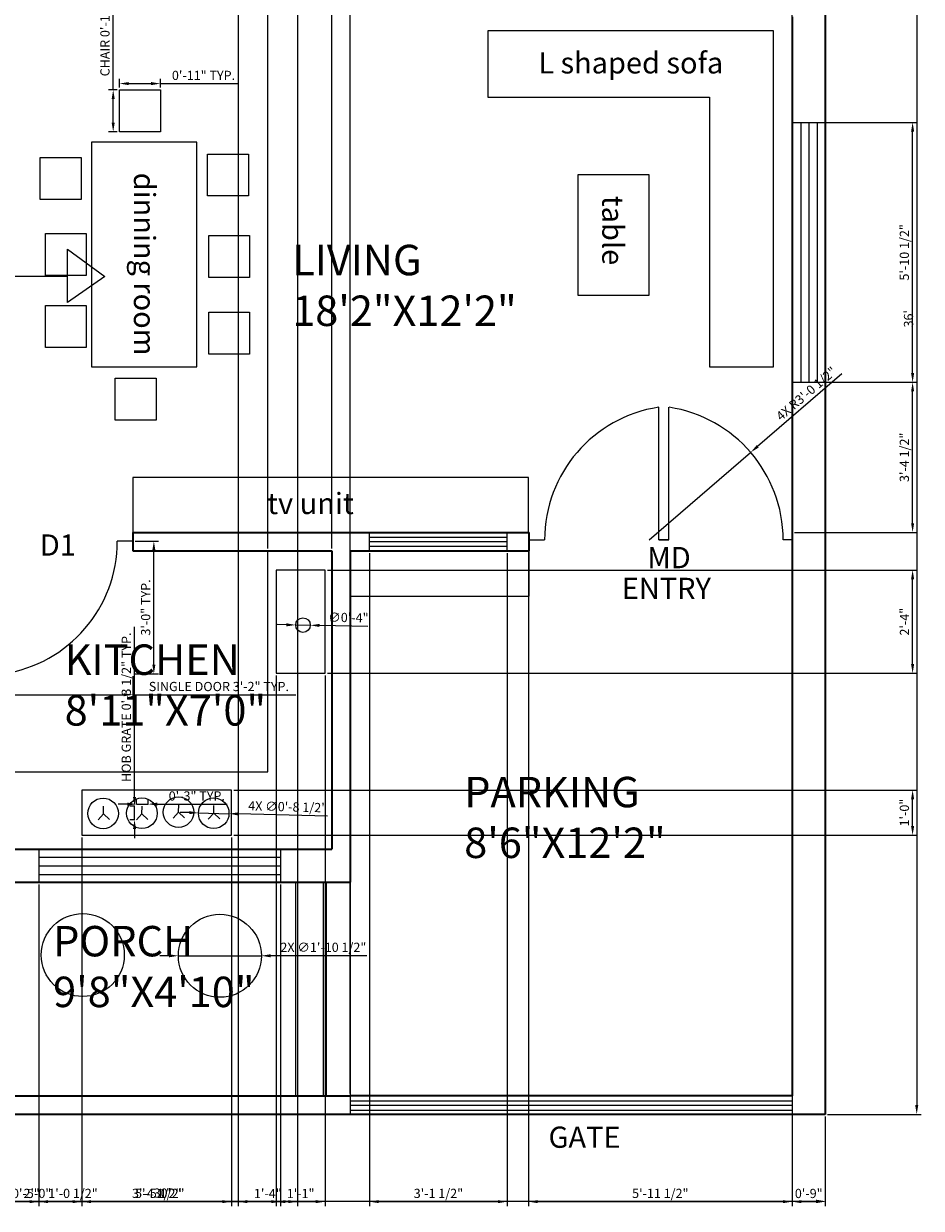
# Model space of a CAD drawing. Units: inches. Extents: x 346 to 762, y 179 to 666.
# Tile 2 of 3: x 518 to 762, y 179 to 500. Entities that reach past the tile are written whole.
import ezdxf

# ---------------------------------------------------------------- set-up
doc = ezdxf.new("R2010")
doc.units = ezdxf.units.IN
for name, color, linetype, lineweight in [('A-ANNO-DIMS', 2, 'Continuous', 18), ('A-ANNO-SYMB', 3, 'Continuous', 18), ('A-ANNO-TEXT', 7, 'Continuous', 18), ('A-AREA-IDEN', 7, 'Continuous', 25), ('A-DOOR', 3, 'Continuous', 25), ('A-EQPM', 8, 'Continuous', 18), ('A-FLOR', 7, 'Continuous', 25), ('A-FLOR-CASE', 9, 'Continuous', 18), ('A-FLOR-FIXT', 9, 'Continuous', 18), ('A-FURN', 8, 'Continuous', 18), ('A-GLAZ', 4, 'Continuous', 18), ('A-WALL', 7, 'Continuous', 35)]:
    doc.layers.add(name, color=color, linetype=linetype, lineweight=lineweight)
doc.styles.get("Standard").update_dxf_attribs({"font": 'arial.ttf'})
doc.dimstyles.new('ISO-25', dxfattribs={"dimtxt": 2.5, "dimasz": 2.5, "dimexe": 1.25, "dimexo": 0.625, "dimtad": 1, "dimdec": 0, "dimlunit": 3, "dimtxsty": 'Standard', "dimcen": 2.5, "dimadec": 0, "dimazin": 0, "dimtfac": 1, "dimtdec": 0, "dimtmove": 0, "dimatfit": 3, "dimfxl": 1, "dimarcsym": 0})

# ---------------------------------------------------------------- blocks, each defined once
blk = doc.blocks.new('*D3')
at = {"layer": 'A-ANNO-DIMS', "color": 0, "lineweight": -2, "transparency": 16777216}
for p, q in [((736.29, 636.22), (761.72, 636.22)), ((760.47, 633.72), (760.47, 206.72)), ((736.29, 204.22), (761.72, 204.22))]:
    blk.add_line(p, q, dxfattribs=at)
at = {"layer": 'A-ANNO-DIMS', "color": 0, "transparency": 16777216}
for points in [[(760.06, 633.72), (760.89, 633.72), (760.47, 636.22)], [(760.06, 206.72), (760.89, 206.72), (760.47, 204.22)]]:
    blk.add_solid(points, dxfattribs=at)
at = {"layer": 'Defpoints', "color": 0, "transparency": 16777216}
for p in [(735.66, 636.22), (735.66, 204.22), (760.47, 204.22)]:
    blk.add_point(p, dxfattribs=at)
at = {"layer": 'A-ANNO-DIMS', "color": 0, "transparency": 16777216, "insert": (758.57, 420.22), "char_height": 2.5, "attachment_point": 5, "rotation": 90}
blk.add_mtext("36'", dxfattribs=at)
blk = doc.blocks.new('*D4')
at = {"layer": 'A-ANNO-DIMS', "color": 0, "lineweight": -2, "transparency": 16777216}
for p, q in [((375.66, 203.6), (375.66, 179.38)), ((735.66, 203.6), (735.66, 179.38)), ((378.16, 180.63), (733.16, 180.63))]:
    blk.add_line(p, q, dxfattribs=at)
at = {"layer": 'A-ANNO-DIMS', "color": 0, "transparency": 16777216}
for points in [[(378.16, 181.05), (378.16, 180.21), (375.66, 180.63)], [(733.16, 181.05), (733.16, 180.21), (735.66, 180.63)]]:
    blk.add_solid(points, dxfattribs=at)
at = {"layer": 'Defpoints', "color": 0, "transparency": 16777216}
for p in [(375.66, 204.22), (735.66, 204.22), (735.66, 180.63)]:
    blk.add_point(p, dxfattribs=at)
at = {"layer": 'A-ANNO-DIMS', "color": 0, "transparency": 16777216, "insert": (555.66, 182.53), "char_height": 2.5, "attachment_point": 5}
blk.add_mtext("30'", dxfattribs=at)
blk = doc.blocks.new('DOOR-SINGLE-36IN')
for p, q in [((2.79, 36), (0, 36)), ((2.79, 36), (2.79, 0)), ((38, 36), (33.78, 36))]:
    blk.add_line(p, q)
blk.add_arc((-2.63, 36), 36.41, 278.5676, 0)
blk = doc.blocks.new('CHAIR-DINING')
blk.add_lwpolyline([(0, 11.39), (11.09, 11.39), (11.09, 0), (0, 0)], close=True)
blk = doc.blocks.new('HOB-PAN-SUPPORT')
for q in [(1.53, 3.67), (0, 0), (3.11, 0.08)]:
    blk.add_line((1.45, 1.6), q)
blk = doc.blocks.new('*D11')
at = {"layer": 'A-ANNO-DIMS', "color": 0, "lineweight": -2, "transparency": 16777216}
for p, q in [((509.66, 323.21), (509.66, 316.88)), ((547.66, 323.21), (547.66, 316.88)), ((512.16, 318.13), (545.16, 318.13)), ((547.66, 318.13), (591.87, 318.13))]:
    blk.add_line(p, q, dxfattribs=at)
at = {"layer": 'A-ANNO-DIMS', "color": 0, "transparency": 16777216}
for points in [[(512.16, 318.55), (512.16, 317.72), (509.66, 318.13)], [(545.16, 318.55), (545.16, 317.72), (547.66, 318.13)]]:
    blk.add_solid(points, dxfattribs=at)
at = {"layer": 'Defpoints', "color": 0, "transparency": 16777216}
for p in [(509.66, 323.83), (547.66, 323.83), (547.66, 318.13)]:
    blk.add_point(p, dxfattribs=at)
at = {"layer": 'A-ANNO-DIMS', "color": 0, "transparency": 16777216, "insert": (571.01, 320.05), "char_height": 2.5, "attachment_point": 5}
blk.add_mtext('SINGLE DOOR 3\'-2" TYP.', dxfattribs=at)
blk = doc.blocks.new('*D12')
at = {"layer": 'A-ANNO-DIMS', "color": 0, "lineweight": -2, "transparency": 16777216}
for p, q in [((548.29, 359.83), (554.61, 359.83)), ((553.36, 326.33), (553.36, 357.33)), ((548.29, 323.83), (554.61, 323.83))]:
    blk.add_line(p, q, dxfattribs=at)
at = {"layer": 'A-ANNO-DIMS', "color": 0, "transparency": 16777216}
for points in [[(552.94, 357.33), (553.78, 357.33), (553.36, 359.83)], [(552.94, 326.33), (553.78, 326.33), (553.36, 323.83)]]:
    blk.add_solid(points, dxfattribs=at)
at = {"layer": 'Defpoints', "color": 0, "transparency": 16777216}
for p in [(547.66, 359.83), (553.36, 359.83), (547.66, 323.83)]:
    blk.add_point(p, dxfattribs=at)
at = {"layer": 'A-ANNO-DIMS', "color": 0, "transparency": 16777216, "insert": (551.46, 341.83), "char_height": 2.5, "attachment_point": 5, "rotation": 90}
blk.add_mtext('3\'-0" TYP.', dxfattribs=at)
blk = doc.blocks.new('*D13')
at = {"layer": 'A-ANNO-DIMS', "color": 0, "lineweight": -2, "transparency": 16777216}
for p, q in [((542.32, 482.35), (542.32, 520.92)), ((543.4, 482.35), (541.07, 482.35)), ((542.32, 473.46), (542.32, 479.85)), ((543.4, 470.96), (541.07, 470.96))]:
    blk.add_line(p, q, dxfattribs=at)
at = {"layer": 'A-ANNO-DIMS', "color": 0, "transparency": 16777216}
for points in [[(541.9, 479.85), (542.74, 479.85), (542.32, 482.35)], [(541.9, 473.46), (542.74, 473.46), (542.32, 470.96)]]:
    blk.add_solid(points, dxfattribs=at)
at = {"layer": 'Defpoints', "color": 0, "transparency": 16777216}
for p in [(542.32, 482.35), (544.03, 482.35), (544.03, 470.96)]:
    blk.add_point(p, dxfattribs=at)
at = {"layer": 'A-ANNO-DIMS', "color": 0, "transparency": 16777216, "insert": (540.4, 502.88), "char_height": 2.5, "attachment_point": 5, "rotation": 90}
blk.add_mtext('CHAIR 0\'-11 1/2" TYP.', dxfattribs=at)
blk = doc.blocks.new('*D14')
at = {"layer": 'A-ANNO-DIMS', "color": 0, "lineweight": -2, "transparency": 16777216}
for p, q in [((544.03, 482.98), (544.03, 485.31)), ((546.53, 484.06), (552.62, 484.06)), ((555.12, 482.98), (555.12, 485.31)), ((555.12, 484.06), (576.05, 484.06))]:
    blk.add_line(p, q, dxfattribs=at)
at = {"layer": 'A-ANNO-DIMS', "color": 0, "transparency": 16777216}
for points in [[(546.53, 484.48), (546.53, 483.64), (544.03, 484.06)], [(552.62, 484.48), (552.62, 483.64), (555.12, 484.06)]]:
    blk.add_solid(points, dxfattribs=at)
at = {"layer": 'Defpoints', "color": 0, "transparency": 16777216}
for p in [(555.12, 484.06), (544.03, 482.35), (555.12, 482.35)]:
    blk.add_point(p, dxfattribs=at)
at = {"layer": 'A-ANNO-DIMS', "color": 0, "transparency": 16777216, "insert": (566.84, 485.96), "char_height": 2.5, "attachment_point": 5}
blk.add_mtext('0\'-11" TYP.', dxfattribs=at)
blk = doc.blocks.new('*D15')
at = {"layer": 'A-ANNO-DIMS', "color": 0, "lineweight": -2, "transparency": 16777216}
for p, q in [((548.11, 290.39), (548.11, 336.61)), ((548.04, 287.89), (546.86, 287.89)), ((548.11, 284.22), (548.11, 287.89)), ((548.04, 284.22), (546.86, 284.22)), ((548.11, 281.72), (548.11, 279.22))]:
    blk.add_line(p, q, dxfattribs=at)
at = {"layer": 'A-ANNO-DIMS', "color": 0, "transparency": 16777216}
for points in [[(547.7, 290.39), (548.53, 290.39), (548.11, 287.89)], [(547.7, 281.72), (548.53, 281.72), (548.11, 284.22)]]:
    blk.add_solid(points, dxfattribs=at)
at = {"layer": 'Defpoints', "color": 0, "transparency": 16777216}
for p in [(548.11, 287.89), (548.66, 287.89), (548.66, 284.22)]:
    blk.add_point(p, dxfattribs=at)
at = {"layer": 'A-ANNO-DIMS', "color": 0, "transparency": 16777216, "insert": (546.19, 314.75), "char_height": 2.5, "attachment_point": 5, "rotation": 90}
blk.add_mtext('HOB GRATE 0\'-3 1/2" TYP.', dxfattribs=at)
blk = doc.blocks.new('*D16')
at = {"layer": 'A-ANNO-DIMS', "color": 0, "lineweight": -2, "transparency": 16777216}
for p, q in [((548.66, 288.51), (548.66, 289.69)), ((551.78, 288.51), (551.78, 289.69)), ((546.16, 288.44), (543.66, 288.44)), ((548.66, 288.44), (551.78, 288.44)), ((554.28, 288.44), (573.26, 288.44))]:
    blk.add_line(p, q, dxfattribs=at)
at = {"layer": 'A-ANNO-DIMS', "color": 0, "transparency": 16777216}
for points in [[(546.16, 288.86), (546.16, 288.02), (548.66, 288.44)], [(554.28, 288.86), (554.28, 288.02), (551.78, 288.44)]]:
    blk.add_solid(points, dxfattribs=at)
at = {"layer": 'Defpoints', "color": 0, "transparency": 16777216}
for p in [(548.66, 287.89), (551.78, 288.44), (551.78, 287.89)]:
    blk.add_point(p, dxfattribs=at)
at = {"layer": 'A-ANNO-DIMS', "color": 0, "transparency": 16777216, "insert": (565.02, 290.34), "char_height": 2.5, "attachment_point": 5}
blk.add_mtext('0\'-3" TYP.', dxfattribs=at)
blk = doc.blocks.new('*D18')
at = {"layer": 'A-ANNO-DIMS', "color": 0, "lineweight": -2, "transparency": 16777216}
for p, q in [((584.3, 357.85), (584.3, 661.17)), ((586.8, 659.92), (599.16, 659.92)), ((601.66, 357.85), (601.66, 661.17))]:
    blk.add_line(p, q, dxfattribs=at)
at = {"layer": 'A-ANNO-DIMS', "color": 0, "transparency": 16777216}
for points in [[(586.8, 660.34), (586.8, 659.51), (584.3, 659.92)], [(599.16, 660.34), (599.16, 659.51), (601.66, 659.92)]]:
    blk.add_solid(points, dxfattribs=at)
at = {"layer": 'Defpoints', "color": 0, "transparency": 16777216}
for p in [(601.66, 659.92), (584.3, 357.22), (601.66, 357.22)]:
    blk.add_point(p, dxfattribs=at)
at = {"layer": 'A-ANNO-DIMS', "color": 0, "transparency": 16777216, "insert": (592.98, 661.84), "char_height": 2.5, "attachment_point": 5}
blk.add_mtext('1\'-5 1/2"', dxfattribs=at)
blk = doc.blocks.new('*D19')
at = {"layer": 'A-ANNO-DIMS', "color": 0, "lineweight": -2, "transparency": 16777216}
for p, q in [((533.83, 279.4), (533.83, 179.27)), ((509.66, 275.6), (509.66, 179.27)), ((512.16, 180.52), (531.33, 180.52))]:
    blk.add_line(p, q, dxfattribs=at)
at = {"layer": 'A-ANNO-DIMS', "color": 0, "transparency": 16777216}
for points in [[(512.16, 180.94), (512.16, 180.11), (509.66, 180.52)], [(531.33, 180.94), (531.33, 180.11), (533.83, 180.52)]]:
    blk.add_solid(points, dxfattribs=at)
at = {"layer": 'Defpoints', "color": 0, "transparency": 16777216}
for p in [(533.83, 280.02), (509.66, 276.22), (533.83, 180.52)]:
    blk.add_point(p, dxfattribs=at)
at = {"layer": 'A-ANNO-DIMS', "color": 0, "transparency": 16777216, "insert": (521.75, 182.42), "char_height": 2.5, "attachment_point": 5}
blk.add_mtext('2\'-0"', dxfattribs=at)
blk = doc.blocks.new('*D20')
at = {"layer": 'A-ANNO-DIMS', "color": 0, "lineweight": -2, "transparency": 16777216}
for p, q in [((533.83, 279.4), (533.83, 179.27)), ((574.44, 279.4), (574.44, 179.27)), ((536.33, 180.52), (571.94, 180.52))]:
    blk.add_line(p, q, dxfattribs=at)
at = {"layer": 'A-ANNO-DIMS', "color": 0, "transparency": 16777216}
for points in [[(536.33, 180.94), (536.33, 180.11), (533.83, 180.52)], [(571.94, 180.94), (571.94, 180.11), (574.44, 180.52)]]:
    blk.add_solid(points, dxfattribs=at)
at = {"layer": 'Defpoints', "color": 0, "transparency": 16777216}
for p in [(533.83, 280.02), (574.44, 280.02), (574.44, 180.52)]:
    blk.add_point(p, dxfattribs=at)
at = {"layer": 'A-ANNO-DIMS', "color": 0, "transparency": 16777216, "insert": (554.13, 182.44), "char_height": 2.5, "attachment_point": 5}
blk.add_mtext('3\'-4 1/2"', dxfattribs=at)
blk = doc.blocks.new('*D21')
at = {"layer": 'A-ANNO-DIMS', "color": 0, "lineweight": -2, "transparency": 16777216}
for p, q in [((575.06, 292.27), (760.61, 292.27)), ((759.36, 282.52), (759.36, 289.77)), ((575.06, 280.02), (760.61, 280.02))]:
    blk.add_line(p, q, dxfattribs=at)
at = {"layer": 'A-ANNO-DIMS', "color": 0, "transparency": 16777216}
for points in [[(758.94, 289.77), (759.78, 289.77), (759.36, 292.27)], [(758.94, 282.52), (759.78, 282.52), (759.36, 280.02)]]:
    blk.add_solid(points, dxfattribs=at)
at = {"layer": 'Defpoints', "color": 0, "transparency": 16777216}
for p in [(574.44, 292.27), (759.36, 292.27), (574.44, 280.02)]:
    blk.add_point(p, dxfattribs=at)
at = {"layer": 'A-ANNO-DIMS', "color": 0, "transparency": 16777216, "insert": (757.46, 286.15), "char_height": 2.5, "attachment_point": 5, "rotation": 90}
blk.add_mtext('1\'-0"', dxfattribs=at)
blk = doc.blocks.new('*D22')
at = {"layer": 'A-ANNO-DIMS', "color": 0, "lineweight": -2, "transparency": 16777216}
for p, q in [((600.46, 351.98), (760.61, 351.98)), ((759.36, 326.47), (759.36, 349.48)), ((600.46, 323.97), (760.61, 323.97))]:
    blk.add_line(p, q, dxfattribs=at)
at = {"layer": 'A-ANNO-DIMS', "color": 0, "transparency": 16777216}
for points in [[(758.94, 349.48), (759.78, 349.48), (759.36, 351.98)], [(758.94, 326.47), (759.78, 326.47), (759.36, 323.97)]]:
    blk.add_solid(points, dxfattribs=at)
at = {"layer": 'Defpoints', "color": 0, "transparency": 16777216}
for p in [(599.83, 351.98), (759.36, 351.98), (599.83, 323.97)]:
    blk.add_point(p, dxfattribs=at)
at = {"layer": 'A-ANNO-DIMS', "color": 0, "transparency": 16777216, "insert": (757.48, 337.97), "char_height": 2.5, "attachment_point": 5, "rotation": 90}
blk.add_mtext('2\'-4"', dxfattribs=at)
blk = doc.blocks.new('*D23')
at = {"layer": 'A-ANNO-DIMS', "color": 0, "lineweight": -2, "transparency": 16777216}
for p, q in [((586.58, 323.34), (586.58, 179.27)), ((599.83, 323.34), (599.83, 179.27)), ((589.08, 180.52), (597.33, 180.52))]:
    blk.add_line(p, q, dxfattribs=at)
at = {"layer": 'A-ANNO-DIMS', "color": 0, "transparency": 16777216}
for points in [[(589.08, 180.94), (589.08, 180.11), (586.58, 180.52)], [(597.33, 180.94), (597.33, 180.11), (599.83, 180.52)]]:
    blk.add_solid(points, dxfattribs=at)
at = {"layer": 'Defpoints', "color": 0, "transparency": 16777216}
for p in [(586.58, 323.97), (599.83, 323.97), (599.83, 180.52)]:
    blk.add_point(p, dxfattribs=at)
at = {"layer": 'A-ANNO-DIMS', "color": 0, "transparency": 16777216, "insert": (593.21, 182.4), "char_height": 2.5, "attachment_point": 5}
blk.add_mtext('1\'-1"', dxfattribs=at)
blk = doc.blocks.new('*D24')
at = {"layer": 'A-ANNO-DIMS', "color": 0, "lineweight": -2, "transparency": 16777216}
for p, q in [((509.66, 266.6), (509.66, 179.27)), ((522.15, 266.6), (522.15, 179.27)), ((512.16, 180.52), (519.65, 180.52)), ((522.15, 180.52), (538.14, 180.52))]:
    blk.add_line(p, q, dxfattribs=at)
at = {"layer": 'A-ANNO-DIMS', "color": 0, "transparency": 16777216}
for points in [[(512.16, 180.94), (512.16, 180.11), (509.66, 180.52)], [(519.65, 180.94), (519.65, 180.11), (522.15, 180.52)]]:
    blk.add_solid(points, dxfattribs=at)
at = {"layer": 'Defpoints', "color": 0, "transparency": 16777216}
for p in [(509.66, 267.22), (522.15, 267.22), (522.15, 180.52)]:
    blk.add_point(p, dxfattribs=at)
at = {"layer": 'A-ANNO-DIMS', "color": 0, "transparency": 16777216, "insert": (531.4, 182.44), "char_height": 2.5, "attachment_point": 5}
blk.add_mtext('1\'-0 1/2"', dxfattribs=at)
blk = doc.blocks.new('*D25')
at = {"layer": 'A-ANNO-DIMS', "color": 0, "lineweight": -2, "transparency": 16777216}
for p, q in [((522.15, 266.6), (522.15, 179.27)), ((587.77, 266.6), (587.77, 179.27)), ((524.65, 180.52), (585.27, 180.52))]:
    blk.add_line(p, q, dxfattribs=at)
at = {"layer": 'A-ANNO-DIMS', "color": 0, "transparency": 16777216}
for points in [[(524.65, 180.94), (524.65, 180.11), (522.15, 180.52)], [(585.27, 180.94), (585.27, 180.11), (587.77, 180.52)]]:
    blk.add_solid(points, dxfattribs=at)
at = {"layer": 'Defpoints', "color": 0, "transparency": 16777216}
for p in [(522.15, 267.22), (587.77, 267.22), (587.77, 180.52)]:
    blk.add_point(p, dxfattribs=at)
at = {"layer": 'A-ANNO-DIMS', "color": 0, "transparency": 16777216, "insert": (554.96, 182.44), "char_height": 2.5, "attachment_point": 5}
blk.add_mtext('5\'-5 1/2"', dxfattribs=at)
blk = doc.blocks.new('*D37')
at = {"layer": 'A-ANNO-DIMS', "color": 0, "lineweight": -2, "transparency": 16777216}
for p, q in [((727.29, 473.5), (760.61, 473.5)), ((759.36, 405.47), (759.36, 471)), ((727.29, 402.97), (760.61, 402.97))]:
    blk.add_line(p, q, dxfattribs=at)
at = {"layer": 'A-ANNO-DIMS', "color": 0, "transparency": 16777216}
for points in [[(758.94, 471), (759.78, 471), (759.36, 473.5)], [(758.94, 405.47), (759.78, 405.47), (759.36, 402.97)]]:
    blk.add_solid(points, dxfattribs=at)
at = {"layer": 'Defpoints', "color": 0, "transparency": 16777216}
for p in [(726.66, 473.5), (759.36, 473.5), (726.66, 402.97)]:
    blk.add_point(p, dxfattribs=at)
at = {"layer": 'A-ANNO-DIMS', "color": 0, "transparency": 16777216, "insert": (757.44, 438.24), "char_height": 2.5, "attachment_point": 5, "rotation": 90}
blk.add_mtext('5\'-10 1/2"', dxfattribs=at)
blk = doc.blocks.new('*D38')
at = {"layer": 'A-ANNO-DIMS', "color": 0, "lineweight": -2, "transparency": 16777216}
for p, q in [((727.29, 402.97), (760.61, 402.97)), ((759.36, 364.72), (759.36, 400.47)), ((727.29, 362.22), (760.61, 362.22))]:
    blk.add_line(p, q, dxfattribs=at)
at = {"layer": 'A-ANNO-DIMS', "color": 0, "transparency": 16777216}
for points in [[(758.94, 400.47), (759.78, 400.47), (759.36, 402.97)], [(758.94, 364.72), (759.78, 364.72), (759.36, 362.22)]]:
    blk.add_solid(points, dxfattribs=at)
at = {"layer": 'Defpoints', "color": 0, "transparency": 16777216}
for p in [(726.66, 402.97), (759.36, 402.97), (726.66, 362.22)]:
    blk.add_point(p, dxfattribs=at)
at = {"layer": 'A-ANNO-DIMS', "color": 0, "transparency": 16777216, "insert": (757.44, 382.6), "char_height": 2.5, "attachment_point": 5, "rotation": 90}
blk.add_mtext('3\'-4 1/2"', dxfattribs=at)
blk = doc.blocks.new('*D39')
at = {"layer": 'A-ANNO-DIMS', "color": 0, "lineweight": -2, "transparency": 16777216}
for p, q in [((606.66, 209.85), (606.66, 661.17)), ((609.16, 659.92), (724.16, 659.92)), ((726.66, 209.85), (726.66, 661.17))]:
    blk.add_line(p, q, dxfattribs=at)
at = {"layer": 'A-ANNO-DIMS', "color": 0, "transparency": 16777216}
for points in [[(609.16, 660.34), (609.16, 659.51), (606.66, 659.92)], [(724.16, 660.34), (724.16, 659.51), (726.66, 659.92)]]:
    blk.add_solid(points, dxfattribs=at)
at = {"layer": 'Defpoints', "color": 0, "transparency": 16777216}
for p in [(726.66, 659.92), (606.66, 209.22), (726.66, 209.22)]:
    blk.add_point(p, dxfattribs=at)
at = {"layer": 'A-ANNO-DIMS', "color": 0, "transparency": 16777216, "insert": (666.66, 661.82), "char_height": 2.5, "attachment_point": 5}
blk.add_mtext('10\'-0"', dxfattribs=at)
blk = doc.blocks.new('*D40')
at = {"layer": 'A-ANNO-DIMS', "color": 0, "lineweight": -2, "transparency": 16777216}
for p, q in [((726.66, 208.6), (726.66, 179.27)), ((735.66, 203.6), (735.66, 179.27)), ((729.16, 180.52), (733.16, 180.52))]:
    blk.add_line(p, q, dxfattribs=at)
at = {"layer": 'A-ANNO-DIMS', "color": 0, "transparency": 16777216}
for points in [[(729.16, 180.94), (729.16, 180.11), (726.66, 180.52)], [(733.16, 180.94), (733.16, 180.11), (735.66, 180.52)]]:
    blk.add_solid(points, dxfattribs=at)
at = {"layer": 'Defpoints', "color": 0, "transparency": 16777216}
for p in [(726.66, 209.22), (735.66, 204.22), (735.66, 180.52)]:
    blk.add_point(p, dxfattribs=at)
at = {"layer": 'A-ANNO-DIMS', "color": 0, "transparency": 16777216, "insert": (731.16, 182.42), "char_height": 2.5, "attachment_point": 5}
blk.add_mtext('0\'-9"', dxfattribs=at)
blk = doc.blocks.new('*D43')
at = {"layer": 'A-ANNO-DIMS', "color": 0, "lineweight": -2, "transparency": 16777216}
for p, q in [((611.94, 356.6), (611.94, 179.27)), ((649.31, 356.6), (649.31, 179.27)), ((614.44, 180.52), (646.81, 180.52))]:
    blk.add_line(p, q, dxfattribs=at)
at = {"layer": 'A-ANNO-DIMS', "color": 0, "transparency": 16777216}
for points in [[(614.44, 180.94), (614.44, 180.11), (611.94, 180.52)], [(646.81, 180.94), (646.81, 180.11), (649.31, 180.52)]]:
    blk.add_solid(points, dxfattribs=at)
at = {"layer": 'Defpoints', "color": 0, "transparency": 16777216}
for p in [(611.94, 357.22), (649.31, 357.22), (649.31, 180.52)]:
    blk.add_point(p, dxfattribs=at)
at = {"layer": 'A-ANNO-DIMS', "color": 0, "transparency": 16777216, "insert": (630.62, 182.44), "char_height": 2.5, "attachment_point": 5}
blk.add_mtext('3\'-1 1/2"', dxfattribs=at)
blk = doc.blocks.new('*D44')
at = {"layer": 'A-ANNO-DIMS', "color": 0, "lineweight": -2, "transparency": 16777216}
for p, q in [((655.05, 361.6), (655.05, 179.27)), ((726.66, 361.6), (726.66, 179.27)), ((657.55, 180.52), (724.16, 180.52))]:
    blk.add_line(p, q, dxfattribs=at)
at = {"layer": 'A-ANNO-DIMS', "color": 0, "transparency": 16777216}
for points in [[(657.55, 180.94), (657.55, 180.11), (655.05, 180.52)], [(724.16, 180.94), (724.16, 180.11), (726.66, 180.52)]]:
    blk.add_solid(points, dxfattribs=at)
at = {"layer": 'Defpoints', "color": 0, "transparency": 16777216}
for p in [(655.05, 362.22), (726.66, 362.22), (726.66, 180.52)]:
    blk.add_point(p, dxfattribs=at)
at = {"layer": 'A-ANNO-DIMS', "color": 0, "transparency": 16777216, "insert": (690.86, 182.44), "char_height": 2.5, "attachment_point": 5}
blk.add_mtext('5\'-11 1/2"', dxfattribs=at)
blk = doc.blocks.new('*D46')
at = {"layer": 'A-ANNO-DIMS', "color": 0, "lineweight": -2, "transparency": 16777216}
for p, q in [((576.21, 585.6), (576.21, 179.27)), ((592.38, 585.6), (592.38, 179.27)), ((578.71, 180.52), (589.88, 180.52))]:
    blk.add_line(p, q, dxfattribs=at)
at = {"layer": 'A-ANNO-DIMS', "color": 0, "transparency": 16777216}
for points in [[(578.71, 180.94), (578.71, 180.11), (576.21, 180.52)], [(589.88, 180.94), (589.88, 180.11), (592.38, 180.52)]]:
    blk.add_solid(points, dxfattribs=at)
at = {"layer": 'Defpoints', "color": 0, "transparency": 16777216}
for p in [(576.21, 586.22), (592.38, 586.22), (592.38, 180.52)]:
    blk.add_point(p, dxfattribs=at)
at = {"layer": 'A-ANNO-DIMS', "color": 0, "transparency": 16777216, "insert": (584.3, 182.4), "char_height": 2.5, "attachment_point": 5}
blk.add_mtext('1\'-4"', dxfattribs=at)
blk = doc.blocks.new('*D47')
at = {"layer": 'A-ANNO-DIMS', "color": 0, "lineweight": -2, "transparency": 16777216}
for p, q in [((504.66, 236.6), (504.66, 179.27)), ((509.66, 231.6), (509.66, 179.27)), ((502.16, 180.52), (499.66, 180.52)), ((504.66, 180.52), (509.66, 180.52)), ((512.16, 180.52), (522.56, 180.52))]:
    blk.add_line(p, q, dxfattribs=at)
at = {"layer": 'A-ANNO-DIMS', "color": 0, "transparency": 16777216}
for points in [[(502.16, 180.94), (502.16, 180.11), (504.66, 180.52)], [(512.16, 180.94), (512.16, 180.11), (509.66, 180.52)]]:
    blk.add_solid(points, dxfattribs=at)
at = {"layer": 'Defpoints', "color": 0, "transparency": 16777216}
for p in [(504.66, 237.22), (509.66, 232.22), (509.66, 180.52)]:
    blk.add_point(p, dxfattribs=at)
at = {"layer": 'A-ANNO-DIMS', "color": 0, "transparency": 16777216, "insert": (518.61, 182.42), "char_height": 2.5, "attachment_point": 5}
blk.add_mtext('0\'-5"', dxfattribs=at)
blk = doc.blocks.new('*D48')
at = {"layer": 'A-ANNO-DIMS', "color": 0, "lineweight": -2, "transparency": 16777216}
for p, q in [((740.13, 405.22), (717.29, 385.56)), ((687.8, 360.18), (715.39, 383.93))]:
    blk.add_line(p, q, dxfattribs=at)
at = {"layer": 'A-ANNO-DIMS', "color": 0, "transparency": 16777216}
blk.add_solid([(717.02, 385.88), (717.56, 385.25), (715.39, 383.93)], dxfattribs=at)
at = {"layer": 'Defpoints', "color": 0, "transparency": 16777216}
for p in [(715.39, 383.93), (687.8, 360.18)]:
    blk.add_point(p, dxfattribs=at)
at = {"layer": 'A-ANNO-DIMS', "color": 0, "transparency": 16777216, "insert": (730.7, 399.63), "char_height": 2.5, "attachment_point": 5, "rotation": 40.716}
blk.add_mtext('4X R3\'-0 1/2"', dxfattribs=at)
blk = doc.blocks.new('*D49')
at = {"layer": 'A-ANNO-DIMS', "color": 0, "lineweight": -2, "transparency": 16777216}
for p, q in [((557.51, 247.27), (555.01, 247.27)), ((560.01, 247.27), (582.54, 247.27)), ((611.21, 247.27), (585.04, 247.27))]:
    blk.add_line(p, q, dxfattribs=at)
at = {"layer": 'A-ANNO-DIMS', "color": 0, "transparency": 16777216}
for points in [[(557.51, 247.69), (557.51, 246.86), (560.01, 247.27)], [(585.04, 247.69), (585.04, 246.86), (582.54, 247.27)]]:
    blk.add_solid(points, dxfattribs=at)
at = {"layer": 'Defpoints', "color": 0, "transparency": 16777216}
for p in [(560.01, 247.27), (582.54, 247.27)]:
    blk.add_point(p, dxfattribs=at)
at = {"layer": 'A-ANNO-DIMS', "color": 0, "transparency": 16777216, "insert": (599.38, 249.25), "char_height": 2.5, "attachment_point": 5, "rotation": 0.0023}
blk.add_mtext('2X ∅1\'-10 1/2"', dxfattribs=at)
blk = doc.blocks.new('*D51')
at = {"layer": 'A-ANNO-DIMS', "color": 0, "lineweight": -2, "transparency": 16777216}
for p, q in [((589.37, 337.12), (586.87, 337.17)), ((591.87, 337.08), (595.83, 337)), ((611.44, 336.7), (598.33, 336.95))]:
    blk.add_line(p, q, dxfattribs=at)
at = {"layer": 'A-ANNO-DIMS', "color": 0, "transparency": 16777216}
for points in [[(589.37, 337.54), (589.36, 336.71), (591.87, 337.08)], [(598.34, 337.37), (598.32, 336.54), (595.83, 337)]]:
    blk.add_solid(points, dxfattribs=at)
at = {"layer": 'Defpoints', "color": 0, "transparency": 16777216}
for p in [(591.87, 337.08), (595.83, 337)]:
    blk.add_point(p, dxfattribs=at)
at = {"layer": 'A-ANNO-DIMS', "color": 0, "transparency": 16777216, "insert": (606.17, 338.77), "char_height": 2.5, "attachment_point": 5, "rotation": 358.898}
blk.add_mtext('∅0\'-4"', dxfattribs=at)
blk = doc.blocks.new('*D52')
at = {"layer": 'A-ANNO-DIMS', "color": 0, "lineweight": -2, "transparency": 16777216}
for p, q in [((562.96, 286.13), (560.46, 286.2)), ((565.46, 286.06), (573.76, 285.85)), ((600.53, 285.15), (576.26, 285.78))]:
    blk.add_line(p, q, dxfattribs=at)
at = {"layer": 'A-ANNO-DIMS', "color": 0, "transparency": 16777216}
for points in [[(562.97, 286.55), (562.95, 285.71), (565.46, 286.06)], [(576.27, 286.2), (576.25, 285.37), (573.76, 285.85)]]:
    blk.add_solid(points, dxfattribs=at)
at = {"layer": 'Defpoints', "color": 0, "transparency": 16777216}
for p in [(565.46, 286.06), (573.76, 285.85)]:
    blk.add_point(p, dxfattribs=at)
at = {"layer": 'A-ANNO-DIMS', "color": 0, "transparency": 16777216, "insert": (589.69, 287.4), "char_height": 2.5, "attachment_point": 5, "rotation": 358.5022}
blk.add_mtext('4X ∅0\'-8 1/2"', dxfattribs=at)

msp = doc.modelspace()

# ---------------------------------------------------------------- linework, layer by layer
at = {"layer": 'A-ANNO-SYMB'}
for p, q in [((529.92, 431.72), (529.92, 439.12)), ((529.92, 439.12), (540.07, 431.72)), ((529.92, 431.72), (402.56, 431.72)), ((540.07, 431.72), (529.92, 424.62)), ((529.92, 424.62), (529.92, 431.72))]:
    msp.add_line(p, q, dxfattribs=at)
at = {"layer": 'A-DOOR'}
for p, q in [((690.43, 360.18), (690.43, 396.18)), ((693.22, 360.18), (693.22, 396.18)), ((655.22, 360.18), (659.45, 360.18)), ((690.43, 360.18), (693.22, 360.18)), ((693.22, 360.18), (690.43, 360.18)), ((726.66, 360.18), (724.21, 360.18)), ((606.66, 209.22), (606.66, 204.22)), ((726.66, 209.22), (726.66, 204.22)), ((606.66, 207.89), (726.66, 207.89)), ((606.66, 206.72), (726.66, 206.72)), ((606.66, 205.35), (726.66, 205.35))]:
    msp.add_line(p, q, dxfattribs=at)
for centre, start, end in [((695.85, 360.18), 98.5676, 180), ((687.8, 360.18), 0, 81.4324)]:
    msp.add_arc(centre, 36.41, start, end, dxfattribs=at)
at = {"layer": 'A-EQPM'}
msp.add_lwpolyline([(533.83, 280.02), (574.44, 280.02), (574.44, 292.27), (533.83, 292.27)], close=True, dxfattribs=at)
for centre in [(539.58, 285.92), (550.12, 285.96), (560.05, 286.26), (569.61, 285.96)]:
    msp.add_circle(centre, 4.15, dxfattribs=at)
at = {"layer": 'A-FLOR'}
for p, q in [((591.86, 267.22), (591.86, 209.22)), ((599.37, 267.22), (599.37, 209.22)), ((600.14, 267.22), (600.14, 209.22)), ((606.66, 267.22), (606.66, 209.22))]:
    msp.add_line(p, q, dxfattribs=at)
msp.add_lwpolyline([(655.22, 357.22), (606.66, 357.22), (606.66, 344.87), (655.22, 344.87)], close=True, dxfattribs=at)
at = {"layer": 'A-FLOR-CASE'}
for p, q in [((584.3, 297.23), (584.3, 357.22)), ((509.66, 297.23), (584.3, 297.23))]:
    msp.add_line(p, q, dxfattribs=at)
msp.add_lwpolyline([(547.66, 362.22), (655.05, 362.22), (655.05, 377.14), (547.66, 377.14)], close=True, dxfattribs=at)
at = {"layer": 'A-FLOR-FIXT'}
for p, q in [((586.58, 351.98), (586.58, 323.97)), ((599.83, 351.98), (586.58, 351.98)), ((599.83, 323.97), (599.83, 351.98)), ((586.58, 323.97), (599.83, 323.97))]:
    msp.add_line(p, q, dxfattribs=at)
msp.add_circle((593.85, 337.04), 1.98, dxfattribs=at)
at = {"layer": 'A-FURN'}
for points in [[(721.6, 480.33), (721.6, 498.42), (643.99, 498.42), (643.99, 480.33), (704.26, 480.33)], [(704.26, 480.33), (704.26, 407.16), (721.6, 407.16), (721.6, 498.42), (704.26, 498.42)]]:
    msp.add_lwpolyline(points, dxfattribs=at)
for points in [[(536.47, 407.16), (565.04, 407.16), (565.04, 468.15), (536.47, 468.15)], [(668.56, 459.38), (687.71, 459.38), (687.71, 426.55), (668.56, 426.55)]]:
    msp.add_lwpolyline(points, close=True, dxfattribs=at)
for centre in [(534.06, 247.48), (571.28, 247.27)]:
    msp.add_circle(centre, 11.27, dxfattribs=at)
at = {"layer": 'A-GLAZ'}
for p, q in [((726.66, 473.5), (735.66, 473.5)), ((729.04, 473.5), (729.04, 402.97)), ((731.16, 473.5), (731.16, 402.97)), ((733.43, 473.5), (733.43, 402.97)), ((726.66, 402.97), (735.66, 402.97)), ((611.94, 357.22), (611.94, 362.22)), ((611.94, 360.93), (649.31, 360.93)), ((649.31, 357.22), (649.31, 362.22)), ((611.94, 359.72), (649.31, 359.72)), ((611.94, 358.46), (649.31, 358.46)), ((522.15, 276.22), (522.15, 267.22)), ((522.15, 274.01), (587.77, 274.01)), ((587.77, 276.22), (587.77, 267.22)), ((522.15, 271.72), (587.77, 271.72)), ((522.15, 269.31), (587.77, 269.31))]:
    msp.add_line(p, q, dxfattribs=at)
at = {"layer": 'A-WALL'}
for p, q in [((735.66, 636.22), (735.66, 204.22)), ((726.66, 502.22), (726.66, 362.22)), ((547.66, 362.22), (655.22, 362.22)), ((547.66, 362.22), (547.66, 357.22)), ((655.22, 357.22), (655.22, 362.22)), ((726.66, 362.22), (726.66, 209.22)), ((547.66, 357.22), (601.66, 357.22)), ((601.66, 357.22), (601.66, 276.22)), ((606.66, 357.22), (606.66, 267.22)), ((606.66, 357.22), (655.22, 357.22)), ((509.66, 276.22), (601.66, 276.22)), ((509.66, 267.22), (606.66, 267.22)), ((509.66, 209.22), (606.66, 209.22)), ((726.66, 209.22), (606.66, 209.22)), ((735.66, 204.22), (375.66, 204.22))]:
    msp.add_line(p, q, dxfattribs=at)

# ---------------------------------------------------------------- block references
at = {"layer": 'A-DOOR'}
msp.add_blockref('DOOR-SINGLE-36IN', (509.66, 323.83), dxfattribs=at)
at = {"layer": 'A-EQPM'}
for p in [(538.2, 284.22), (548.66, 284.22), (558.6, 284.66), (568.15, 284.36)]:
    msp.add_blockref('HOB-PAN-SUPPORT', p, dxfattribs=at)
at = {"layer": 'A-FURN'}
for p in [(544.03, 470.96), (522.53, 452.58), (567.95, 453.55), (523.9, 432), (568.27, 431.43), (523.9, 412.39), (568.27, 410.6), (542.88, 392.71)]:
    msp.add_blockref('CHAIR-DINING', p, dxfattribs=at)

# ---------------------------------------------------------------- texts
at = {"layer": 'A-ANNO-TEXT', "attachment_point": 1}
for s, insert, char_height in [('L shaped sofa', (657.75, 492.57), 5.7635), ('tv unit', (584.11, 372.95), 5.764), ('D1', (522.41, 361.67), 5.764), ('MD', (687.32, 358.25), 5.764), ('ENTRY', (680.4, 349.9), 5.764), ('GATE', (660.51, 200.9), 5.764)]:
    msp.add_mtext_dynamic_manual_height_columns(s, width=202.5556, gutter_width=28.82, heights=[0], dxfattribs=dict(at, insert=insert, char_height=char_height))
at = {"layer": 'A-ANNO-TEXT', "insert": (680.86, 453.61), "char_height": 5.764, "attachment_point": 1, "rotation": 270}
msp.add_mtext_dynamic_manual_height_columns('table', width=202.5556, gutter_width=28.82, heights=[0], dxfattribs=at)
at = {"layer": 'A-AREA-IDEN', "insert": (553.71, 459.88), "char_height": 5.7635, "attachment_point": 1, "rotation": 270}
msp.add_mtext_dynamic_manual_height_columns('dinning room', width=202.5556, gutter_width=28.82, heights=[0], dxfattribs=at)
at = {"layer": 'A-AREA-IDEN', "attachment_point": 1}
for s, insert, char_height in [('LIVING\\P18\'2"X12\'2"', (590.92, 440.29), 8.2632), ('KITCHEN\\P8\'11"X7\'0"', (529.14, 331.8), 8.263), ('PARKING\\P8\'6"X12\'2"', (637.62, 295.85), 8.263), ('PORCH\\P9\'8"X4\'10"', (526.01, 255.37), 8.263)]:
    msp.add_mtext_dynamic_manual_height_columns(s, width=290.4031, gutter_width=41.32, heights=[0], dxfattribs=dict(at, insert=insert, char_height=char_height))

# ---------------------------------------------------------------- dimensions: what is measured, and where the dimension line sits
at = {"layer": 'A-ANNO-DIMS'}
for base, p1, p2, override, picture, middle in [((601.66, 659.92), (584.3, 357.22), (601.66, 357.22), {"dimdec": 1, "dimlfac": 1, "dimrnd": 0, "dimzin": 1, "dimdsep": 46, "dimlunit": 4, "dimfrac": 2}, '*D18', (592.98, 661.84)), ((726.66, 659.92), (606.66, 209.22), (726.66, 209.22), {"dimdec": 1, "dimlfac": 1, "dimrnd": 0, "dimzin": 1, "dimdsep": 46, "dimlunit": 4, "dimfrac": 2}, '*D39', (666.66, 661.82)), ((592.38, 180.52), (576.21, 586.22), (592.38, 586.22), {"dimdec": 1, "dimlfac": 1, "dimrnd": 0, "dimzin": 1, "dimdsep": 46, "dimlunit": 4, "dimfrac": 2}, '*D46', (584.3, 182.4)), ((726.66, 180.52), (655.05, 362.22), (726.66, 362.22), {"dimdec": 1, "dimlfac": 1, "dimrnd": 0, "dimzin": 1, "dimdsep": 46, "dimlunit": 4, "dimfrac": 2}, '*D44', (690.86, 182.44)), ((649.31, 180.52), (611.94, 357.22), (649.31, 357.22), {"dimdec": 1, "dimlfac": 1, "dimrnd": 0, "dimzin": 1, "dimdsep": 46, "dimlunit": 4, "dimfrac": 2}, '*D43', (630.62, 182.44)), ((599.8303, 180.5219), (586.581, 323.9652), (599.8303, 323.9652), {"dimdec": 1, "dimlfac": 1, "dimrnd": 0, "dimzin": 1, "dimdsep": 46, "dimlunit": 4, "dimfrac": 2}, '*D23', (593.2056, 182.402)), ((533.83, 180.52), (509.66, 276.22), (533.83, 280.02), {"dimdec": 1, "dimlfac": 1, "dimrnd": 0, "dimzin": 1, "dimdsep": 46, "dimlunit": 4, "dimfrac": 2}, '*D19', (521.75, 182.42)), ((574.44, 180.52), (533.83, 280.02), (574.44, 280.02), {"dimdec": 1, "dimlfac": 1, "dimrnd": 0, "dimzin": 1, "dimdsep": 46, "dimlunit": 4, "dimfrac": 2}, '*D20', (554.13, 182.44)), ((522.15, 180.52), (509.66, 267.22), (522.15, 267.22), {"dimdec": 1, "dimlfac": 1, "dimrnd": 0, "dimzin": 1, "dimdsep": 46, "dimlunit": 4, "dimfrac": 2}, '*D24', (531.4, 182.44)), ((587.77, 180.52), (522.15, 267.22), (587.77, 267.22), {"dimdec": 1, "dimlfac": 1, "dimrnd": 0, "dimzin": 1, "dimdsep": 46, "dimlunit": 4, "dimfrac": 2}, '*D25', (554.96, 182.44)), ((509.66, 180.52), (504.66, 237.22), (509.66, 232.22), {"dimdec": 1, "dimlfac": 1, "dimrnd": 0, "dimzin": 1, "dimdsep": 46, "dimlunit": 4, "dimfrac": 2}, '*D47', (518.61, 182.42)), ((735.66, 180.52), (726.66, 209.22), (735.66, 204.22), {"dimdec": 1, "dimlfac": 1, "dimrnd": 0, "dimzin": 1, "dimdsep": 46, "dimlunit": 4, "dimfrac": 2}, '*D40', (731.16, 182.42)), ((735.66, 180.63), (375.66, 204.22), (735.66, 204.22), {"dimclrd": 0, "dimclre": 0, "dimclrt": 0}, '*D4', (555.66, 182.53))]:
    dim = msp.add_linear_dim(base=base, p1=p1, p2=p2, dimstyle='ISO-25', override=override, dxfattribs=at)
    dim.commit()
    dim.dimension.update_dxf_attribs({"geometry": picture, "text_midpoint": middle})
for base, p1, p2, override, picture, middle in [((760.47, 204.22), (735.66, 636.22), (735.66, 204.22), {"dimclrd": 0, "dimclre": 0, "dimclrt": 0}, '*D3', (758.57, 420.22)), ((759.36, 473.5), (726.66, 402.97), (726.66, 473.5), {"dimdec": 1, "dimlfac": 1, "dimrnd": 0, "dimzin": 1, "dimdsep": 46, "dimlunit": 4, "dimfrac": 2}, '*D37', (757.44, 438.24)), ((759.3612, 402.9714), (726.6612, 362.2219), (726.6612, 402.9714), {"dimdec": 1, "dimlfac": 1, "dimrnd": 0, "dimzin": 1, "dimdsep": 46, "dimlunit": 4, "dimfrac": 2}, '*D38', (757.4428, 382.5966)), ((759.36, 351.98), (599.83, 323.97), (599.83, 351.98), {"dimdec": 1, "dimlfac": 1, "dimrnd": 0, "dimzin": 1, "dimdsep": 46, "dimlunit": 4, "dimfrac": 2}, '*D22', (757.48, 337.97)), ((759.3612, 292.2655), (574.4372, 280.0247), (574.4372, 292.2655), {"dimdec": 1, "dimlfac": 1, "dimrnd": 0, "dimzin": 1, "dimdsep": 46, "dimlunit": 4, "dimfrac": 2}, '*D21', (757.4598, 286.1451))]:
    dim = msp.add_linear_dim(base=base, p1=p1, p2=p2, angle=90, dimstyle='ISO-25', override=override, dxfattribs=at)
    dim.commit()
    dim.dimension.update_dxf_attribs({"geometry": picture, "text_midpoint": middle})
for base, p1, p2, text, picture, middle in [((542.32, 482.35), (544.03, 470.96), (544.03, 482.35), 'CHAIR <> TYP.', '*D13', (540.4, 502.88)), ((553.36, 359.83), (547.66, 323.83), (547.66, 359.83), '<> TYP.', '*D12', (551.46, 341.83)), ((548.11, 287.89), (548.66, 284.22), (548.66, 287.89), 'HOB GRATE <> TYP.', '*D15', (546.19, 314.75))]:
    dim = msp.add_linear_dim(base=base, p1=p1, p2=p2, angle=90, text=text, dimstyle='ISO-25', override={"dimdec": 1, "dimlfac": 1, "dimrnd": 0, "dimzin": 1, "dimdsep": 46, "dimlunit": 4, "dimfrac": 2}, dxfattribs=at)
    dim.commit()
    dim.dimension.update_dxf_attribs({"geometry": picture, "text_midpoint": middle})
for base, p1, p2, text, picture, middle in [((555.12, 484.06), (544.03, 482.35), (555.12, 482.35), '<> TYP.', '*D14', (566.84, 485.96)), ((547.66, 318.13), (509.66, 323.83), (547.66, 323.83), 'SINGLE DOOR <> TYP.', '*D11', (571.01, 320.05)), ((551.78, 288.44), (548.66, 287.89), (551.78, 287.89), '<> TYP.', '*D16', (565.02, 290.34))]:
    dim = msp.add_linear_dim(base=base, p1=p1, p2=p2, text=text, dimstyle='ISO-25', override={"dimdec": 1, "dimlfac": 1, "dimrnd": 0, "dimzin": 1, "dimdsep": 46, "dimlunit": 4, "dimfrac": 2}, dxfattribs=at)
    dim.commit()
    dim.dimension.update_dxf_attribs({"geometry": picture, "text_midpoint": middle})
dim = msp.add_radius_dim(center=(687.8, 360.18), mpoint=(715.39, 383.93), text='4X <>', dimstyle='ISO-25', override={"dimdec": 1, "dimlfac": 1, "dimrnd": 0, "dimzin": 1, "dimdsep": 46, "dimlunit": 4, "dimfrac": 2}, dxfattribs=at)
dim.commit()
dim.dimension.update_dxf_attribs({"geometry": '*D48', "text_midpoint": (731.95, 398.18), "dimtype": 164})
dim = msp.add_diameter_dim_2p(p1=(591.87, 337.08), p2=(595.83, 337), dimstyle='ISO-25', override={"dimdec": 1, "dimlfac": 1, "dimrnd": 0, "dimzin": 1, "dimdsep": 46, "dimlunit": 4, "dimfrac": 2}, dxfattribs=at)
dim.commit()
dim.dimension.update_dxf_attribs({"geometry": '*D51', "text_midpoint": (606.14, 336.8), "dimtype": 163})
for p1, p2, text, picture, middle in [((565.46, 286.06), (573.76, 285.85), '4X <>', '*D52', (589.64, 285.43)), ((560.01, 247.27), (582.54, 247.27), '2X <>', '*D49', (599.38, 247.27))]:
    dim = msp.add_diameter_dim_2p(p1=p1, p2=p2, text=text, dimstyle='ISO-25', override={"dimdec": 1, "dimlfac": 1, "dimrnd": 0, "dimzin": 1, "dimdsep": 46, "dimlunit": 4, "dimfrac": 2}, dxfattribs=at)
    dim.commit()
    dim.dimension.update_dxf_attribs({"geometry": picture, "text_midpoint": middle, "dimtype": 163})

doc.saveas('drawing.dxf')
